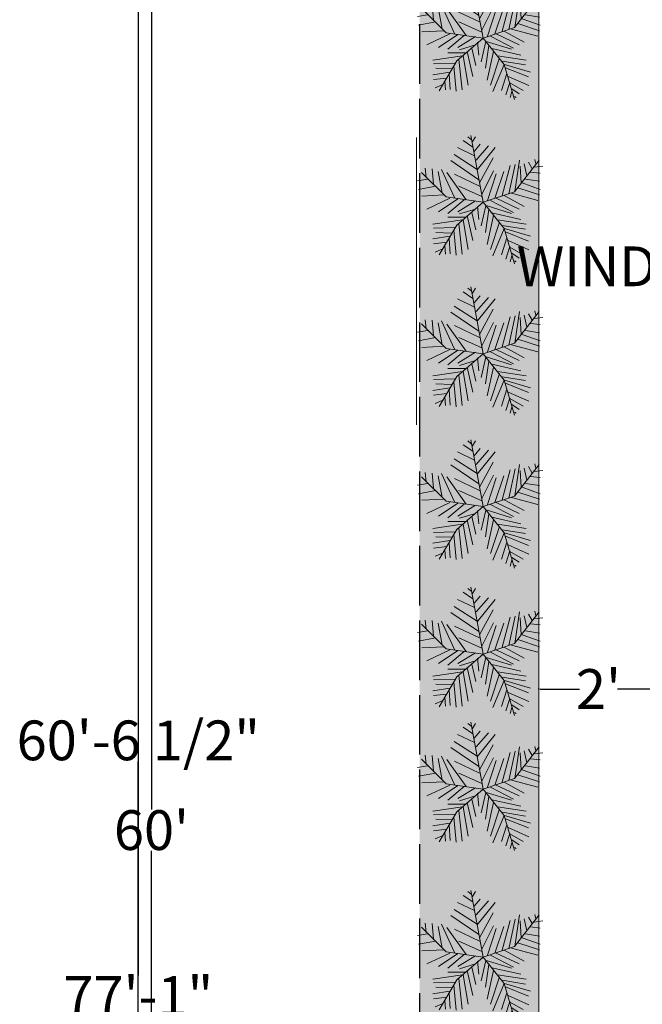
# Model space of a CAD drawing. Units: inches. Extents: x 853 to 1550, y 485 to 1596.
# Tile 3 of 18: x 853 to 979, y 1010 to 1208. Entities that reach past the tile are written whole.
import ezdxf

# ---------------------------------------------------------------- set-up
doc = ezdxf.new("R2010")
doc.units = ezdxf.units.IN
doc.header["$MEASUREMENT"] = 0
doc.linetypes.add('ACAD_ISO02W100', pattern=[15, 12, -3])
for name, color, linetype, lineweight in [('A-ANNO-DIMS', 2, 'Continuous', 18), ('C-PROP', 8, 'ACAD_ISO02W100', 25), ('furniture', 250, 'Continuous', 18), ('L-PLNT-TREE', 106, 'Continuous', 13), ('lawn', 106, 'Continuous', 18)]:
    doc.layers.add(name, color=color, linetype=linetype, lineweight=lineweight)
doc.layers.add('L-PLNT-PATT', color=85, linetype='Continuous', lineweight=13, true_color=0x58ba48)
doc.styles.get("Standard").update_dxf_attribs({"font": 'arial.ttf'})
doc.dimstyles.get("Standard").update_dxf_attribs({"dimtxt": 8, "dimasz": 0.18, "dimexe": 0.18, "dimexo": 0.0625, "dimgap": 0.09, "dimtad": 0, "dimtih": 1, "dimtoh": 1, "dimzin": 0, "dimdsep": 46, "dimlunit": 3, "dimtxsty": 'Standard', "dimcen": 0.09, "dimadec": 0, "dimazin": 0, "dimtfac": 1, "dimtofl": 0, "dimtmove": 0, "dimatfit": 3, "dimfxl": 1, "dimtolj": 1, "dimtzin": 0, "dimarcsym": 0})

# ---------------------------------------------------------------- blocks, each defined once
blk = doc.blocks.new('*U18')
for p, q in [((-8.737, 47.138), (-17.069, 52.711)), ((-10.186, 53.64), (-13.084, 55.962)), ((0, 0), (-10.5, 57)), ((-9.099, 51.782), (-6.563, 55.962)), ((-7.288, 39.707), (-21.778, 46.673)), ((-7.65, 43.423), (-2.578, 49.46)), ((-5.839, 35.992), (4.667, 48.067)), ((-5.114, 27.632), (10.463, 46.673)), ((-3.665, 19.273), (-27.574, 35.527)), ((-5.114, 28.097), (-24.676, 40.636)), ((-2.941, 16.486), (8.652, 37.85)), ((27, 9), (48, 36)), ((27.127, 9.056), (31.112, 35.992)), ((38.719, 34.134), (41.979, 28.561)), ((44.153, 36.456), (45.239, 32.741)), ((-31.5, 4.5), (-52.5, 25.5)), ((-48.585, 21.131), (-49.309, 29.026)), ((-43.513, 28.561), (-42.427, 15.558)), ((-38.442, 26.239), (-34.819, 7.663)), ((-35.544, 28.097), (-24.314, 3.947)), ((-14.533, 2.09), (-30.834, 25.31)), ((-1.129, 6.734), (9.014, 26.704)), ((10.101, 3.483), (17.708, 26.239)), ((16.259, 5.805), (23.142, 31.348)), ((22.055, 7.198), (27.489, 32.277)), ((31.836, 30.883), (32.561, 16.486)), ((35.096, 32.741), (37.27, 22.524)), ((40.53, 25.775), (48.862, 24.846)), ((43.791, 29.954), (51.036, 30.883)), ((-47.498, 19.737), (-55.83, 18.344)), ((-24.314, 23.917), (-2.941, 13.7)), ((3.942, 1.625), (11.187, 24.381)), ((36.183, 19.737), (48.137, 17.88)), ((-40.615, 13.7), (-55.105, 10.913)), ((-20.691, 13.7), (-1.129, 4.876)), ((0, 0), (27, 9)), ((29.662, 12.307), (48.137, 6.269)), ((33.285, 16.486), (48.862, 10.913)), ((-33.37, 6.269), (-52.207, 5.34)), ((-28.299, 3.483), (-47.86, -5.805)), ((-21.416, 3.018), (-38.079, -8.128)), ((0, 0), (-31.5, 4.5)), ((-15.982, 2.09), (-30.11, -9.521)), ((0, 0), (-22.5, -19.5)), ((-6.563, 1.161), (-21.416, -8.128)), ((0, 0), (18, -22.5)), ((6.478, 1.625), (26.04, -8.592)), ((11.187, 3.483), (30.749, -5.805)), ((18.07, 5.805), (35.096, -3.483)), ((24.229, 7.663), (46.688, 1.625)), ((-6.563, -5.805), (-19.967, -9.985)), ((-4.752, -3.483), (-3.665, -14.629)), ((2.493, -3.019), (-1.491, -20.202)), ((1.769, -2.555), (24.229, -9.521)), ((5.029, -6.27), (2.131, -25.775)), ((-17.431, -15.094), (-42.789, -18.809)), ((-15.257, -12.772), (-30.11, -12.772)), ((-17.069, -15.094), (-12.721, -40.172)), ((-13.446, -11.378), (-8.737, -32.741)), ((-9.461, -8.592), (-6.201, -23.453)), ((9.014, -11.378), (3.58, -35.992)), ((7.565, -9.056), (32.198, -14.629)), ((12.274, -15.094), (36.907, -18.809)), ((-24.314, -21.596), (-42.427, -22.06)), ((-22.5, -19.5), (-37.5, -45)), ((-25.038, -23.918), (-22.865, -45.281)), ((-20.691, -18.345), (-17.793, -44.352)), ((14.085, -16.951), (6.478, -40.172)), ((18.07, -22.524), (8.289, -45.745)), ((16.259, -19.738), (36.183, -22.989)), ((18, -22.5), (27, -52.5)), ((18.433, -22.524), (40.53, -29.026)), ((-28.299, -29.026), (-42.789, -31.348)), ((-26.849, -26.24), (-40.253, -25.775)), ((-29.023, -30.884), (-27.936, -43.887)), ((20.244, -30.419), (15.897, -44.816)), ((19.157, -25.311), (38.719, -33.206)), ((21.331, -32.741), (39.081, -40.636)), ((-30.834, -34.135), (-42.427, -35.528)), ((-34.457, -39.708), (-40.978, -42.494)), ((-32.646, -36.921), (-31.921, -44.352)), ((22.78, -37.85), (19.519, -48.532)), ((22.78, -38.314), (34.372, -44.816)), ((24.591, -45.745), (23.142, -50.854)), ((24.591, -43.423), (30.749, -47.603)), ((26.764, -49.925), (28.213, -50.854))]:
    blk.add_line(p, q)
blk = doc.blocks.new('*D21')
at = {"layer": 'A-ANNO-DIMS', "color": 0, "lineweight": -2, "transparency": 16777216}
for p, q in [((957.94, 1073.4), (957.94, 1073.52)), ((958.12, 1073.34), (966.1, 1073.34)), ((981.76, 1073.34), (973.78, 1073.34)), ((981.94, 1073.4), (981.94, 1073.52))]:
    blk.add_line(p, q, dxfattribs=at)
at = {"layer": 'A-ANNO-DIMS', "color": 0, "transparency": 16777216}
for points in [[(958.12, 1073.37), (958.12, 1073.31), (957.94, 1073.34)], [(981.76, 1073.37), (981.76, 1073.31), (981.94, 1073.34)]]:
    blk.add_solid(points, dxfattribs=at)
at = {"layer": 'Defpoints', "color": 0, "transparency": 16777216}
for p in [(957.94, 1073.34), (957.94, 1073.34), (981.94, 1073.34)]:
    blk.add_point(p, dxfattribs=at)
at = {"layer": 'A-ANNO-DIMS', "color": 0, "transparency": 16777216, "insert": (969.94, 1073.34), "char_height": 8, "attachment_point": 5}
blk.add_mtext("\\A1;2'", dxfattribs=at)
blk = doc.blocks.new('*D23')
at = {"layer": 'A-ANNO-DIMS', "color": 0, "lineweight": -2, "transparency": 16777216}
for p, q in [((879.97, 1474.13), (879.75, 1474.13)), ((879.93, 1473.95), (879.93, 1049.11)), ((879.93, 615.92), (879.93, 1040.76)), ((879.97, 615.74), (879.75, 615.74))]:
    blk.add_line(p, q, dxfattribs=at)
at = {"layer": 'A-ANNO-DIMS', "color": 0, "transparency": 16777216}
for points in [[(879.9, 1473.95), (879.96, 1473.95), (879.93, 1474.13)], [(879.9, 615.92), (879.96, 615.92), (879.93, 615.74)]]:
    blk.add_solid(points, dxfattribs=at)
at = {"layer": 'Defpoints', "color": 0, "transparency": 16777216}
for p in [(880.03, 1474.13), (879.93, 615.74), (880.03, 615.74)]:
    blk.add_point(p, dxfattribs=at)
at = {"layer": 'A-ANNO-DIMS', "color": 0, "transparency": 16777216, "insert": (879.93, 1044.94), "char_height": 8, "attachment_point": 5}
blk.add_mtext("\\A1;60'", dxfattribs=at)
blk = doc.blocks.new('*D55')
at = {"layer": 'A-ANNO-DIMS', "color": 0, "lineweight": -2, "transparency": 16777216}
for p, q in [((991, 1205.54), (1005.25, 1205.54)), ((1005.07, 1205.36), (1005.07, 1162.64)), ((1005.07, 1111.47), (1005.07, 1154.18)), ((991, 1111.29), (1005.25, 1111.29))]:
    blk.add_line(p, q, dxfattribs=at)
at = {"layer": 'A-ANNO-DIMS', "color": 0, "transparency": 16777216}
for points in [[(1005.04, 1205.36), (1005.1, 1205.36), (1005.07, 1205.54)], [(1005.04, 1111.47), (1005.1, 1111.47), (1005.07, 1111.29)]]:
    blk.add_solid(points, dxfattribs=at)
at = {"layer": 'Defpoints', "color": 0, "transparency": 16777216}
for p in [(990.94, 1205.54), (1005.07, 1205.54), (990.94, 1111.29)]:
    blk.add_point(p, dxfattribs=at)
at = {"layer": 'A-ANNO-DIMS', "color": 0, "transparency": 16777216, "insert": (1005.07, 1158.41), "char_height": 8, "attachment_point": 5}
blk.add_mtext('\\A1;WINDOW 7\'-10" TYP.', dxfattribs=at)
blk = doc.blocks.new('*D70')
at = {"layer": 'A-ANNO-DIMS', "color": 0, "lineweight": -2, "transparency": 16777216}
for p, q in [((981.87, 1426.13), (877.09, 1426.13)), ((877.27, 1425.95), (877.27, 1067.22)), ((877.27, 700.05), (877.27, 1058.77)), ((1110.88, 699.87), (877.09, 699.87))]:
    blk.add_line(p, q, dxfattribs=at)
at = {"layer": 'A-ANNO-DIMS', "color": 0, "transparency": 16777216}
for points in [[(877.24, 1425.95), (877.3, 1425.95), (877.27, 1426.13)], [(877.24, 700.05), (877.3, 700.05), (877.27, 699.87)]]:
    blk.add_solid(points, dxfattribs=at)
at = {"layer": 'Defpoints', "color": 0, "transparency": 16777216}
for p in [(981.94, 1426.13), (877.27, 699.87), (1110.94, 699.87)]:
    blk.add_point(p, dxfattribs=at)
at = {"layer": 'A-ANNO-DIMS', "color": 0, "transparency": 16777216, "insert": (877.27, 1063), "char_height": 8, "attachment_point": 5}
blk.add_mtext('\\A1;60\'-6 1/2"', dxfattribs=at)
blk = doc.blocks.new('*D71')
at = {"layer": 'A-ANNO-DIMS', "color": 0, "lineweight": -2, "transparency": 16777216}
for p, q in [((933.87, 1474.13), (877.09, 1474.13)), ((877.27, 1473.95), (877.27, 1015.66)), ((877.27, 549.16), (877.27, 1007.45)), ((933.87, 548.98), (877.09, 548.98))]:
    blk.add_line(p, q, dxfattribs=at)
at = {"layer": 'A-ANNO-DIMS', "color": 0, "transparency": 16777216}
for points in [[(877.24, 1473.95), (877.3, 1473.95), (877.27, 1474.13)], [(877.24, 549.16), (877.3, 549.16), (877.27, 548.98)]]:
    blk.add_solid(points, dxfattribs=at)
at = {"layer": 'Defpoints', "color": 0, "transparency": 16777216}
for p in [(877.27, 1474.13), (933.94, 1474.13), (933.94, 548.98)]:
    blk.add_point(p, dxfattribs=at)
at = {"layer": 'A-ANNO-DIMS', "color": 0, "transparency": 16777216, "insert": (877.27, 1011.55), "char_height": 8, "attachment_point": 5}
blk.add_mtext('\\A1;77\'-1"', dxfattribs=at)

msp = doc.modelspace()

# ---------------------------------------------------------------- hatches: boundary and pattern name
at = {"layer": 'L-PLNT-PATT'}
h = msp.add_hatch(color=256, dxfattribs=at)
h.dxf.hatch_style = 1
h.paths.add_polyline_path([(1461.937, 1474.129), (933.937, 1474.129), (933.937, 730.129), (933.937, 622.891), (941.686, 622.891), (941.686, 604.895), (957.937, 604.895), (957.937, 1450.129), (1437.937, 1450.129), (1437.937, 604.895), (1454.646, 604.895), (1454.646, 622.891), (1461.937, 622.891), (1461.937, 734.988)])

# ---------------------------------------------------------------- linework, layer by layer
at = {"layer": 'C-PROP'}
msp.add_line((933.937, 730.129), (933.937, 1474.129), dxfattribs=at)
at = {"layer": 'furniture'}
msp.add_line((933.264, 1126.49), (933.264, 1184.324), dxfattribs=at)
at = {"layer": 'lawn'}
msp.add_line((957.937, 765.455), (957.937, 1450.129), dxfattribs=at)

# ---------------------------------------------------------------- block references
at = {"layer": 'L-PLNT-TREE', "xscale": 0.2357951711934384, "yscale": 0.2357951711934384, "zscale": 0.2357951711934384}
for p in [(946.691, 1204.359), (946.691, 1171.302), (946.691, 1140.83), (946.691, 1110.062), (946.691, 1080.376), (946.691, 1053.196), (946.691, 1019.378)]:
    msp.add_blockref('*U18', p, dxfattribs=at)

# ---------------------------------------------------------------- dimensions: what is measured, and where the dimension line sits
at = {"layer": 'A-ANNO-DIMS'}
for base, p1, p2, picture, middle in [((877.2718, 1474.1293), (933.9371, 548.9788), (933.9371, 1474.1293), '*D71', (877.2718, 1011.5541)), ((877.272, 699.868), (981.937, 1426.129), (1110.94, 699.868), '*D70', (877.272, 1062.999))]:
    dim = msp.add_linear_dim(base=base, p1=p1, p2=p2, angle=90, dimstyle='Standard', override={"dimdec": 1, "dimlfac": 1, "dimrnd": 0, "dimzin": 1, "dimdsep": 46, "dimlunit": 4, "dimfrac": 2}, dxfattribs=at)
    dim.commit()
    dim.dimension.update_dxf_attribs({"geometry": picture, "text_midpoint": middle})
for base, p1, p2, text, override, picture, middle in [((879.933, 615.743), (880.035, 1474.129), (880.035, 615.743), "60'", {"dimclrd": 0, "dimclre": 0, "dimclrt": 0}, '*D23', (879.933, 1044.936)), ((1005.074, 1205.535), (990.937, 1111.29), (990.937, 1205.535), 'WINDOW <> TYP.', {"dimdec": 1, "dimlfac": 1, "dimrnd": 0, "dimzin": 1, "dimdsep": 46, "dimlunit": 4, "dimfrac": 2}, '*D55', (1005.074, 1158.413))]:
    dim = msp.add_linear_dim(base=base, p1=p1, p2=p2, angle=90, text=text, dimstyle='Standard', override=override, dxfattribs=at)
    dim.commit()
    dim.dimension.update_dxf_attribs({"geometry": picture, "text_midpoint": middle})
dim = msp.add_linear_dim(base=(957.937, 1073.341), p1=(981.937, 1073.341), p2=(957.937, 1073.341), dimstyle='Standard', override={"dimclrd": 0, "dimclre": 0, "dimclrt": 0}, dxfattribs=at)
dim.commit()
dim.dimension.update_dxf_attribs({"geometry": '*D21', "text_midpoint": (969.937, 1073.341)})

doc.saveas('drawing.dxf')
